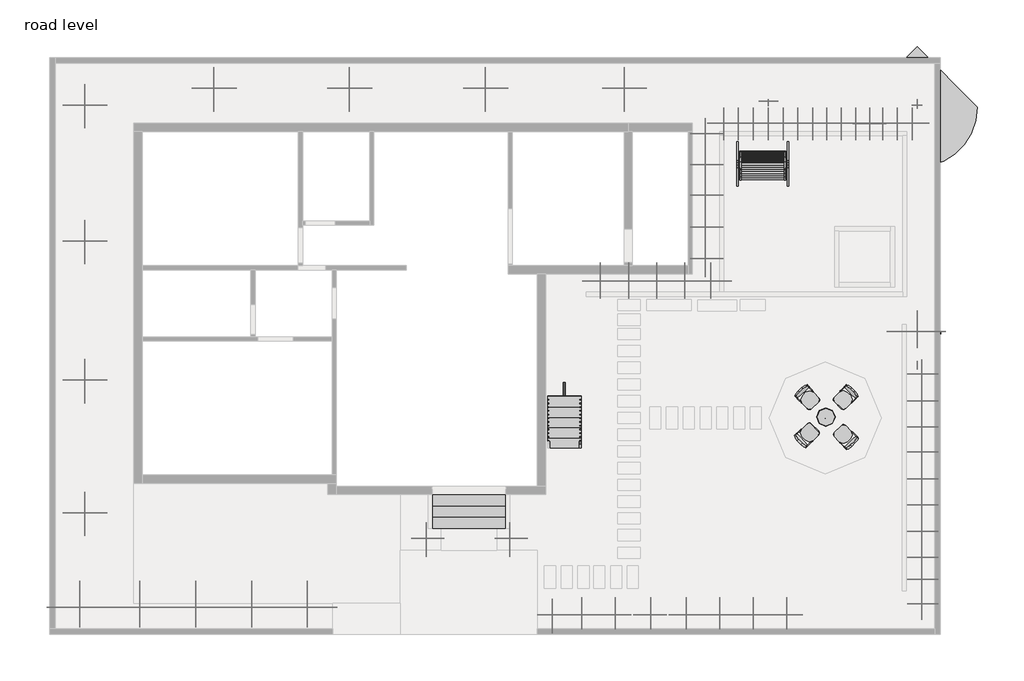
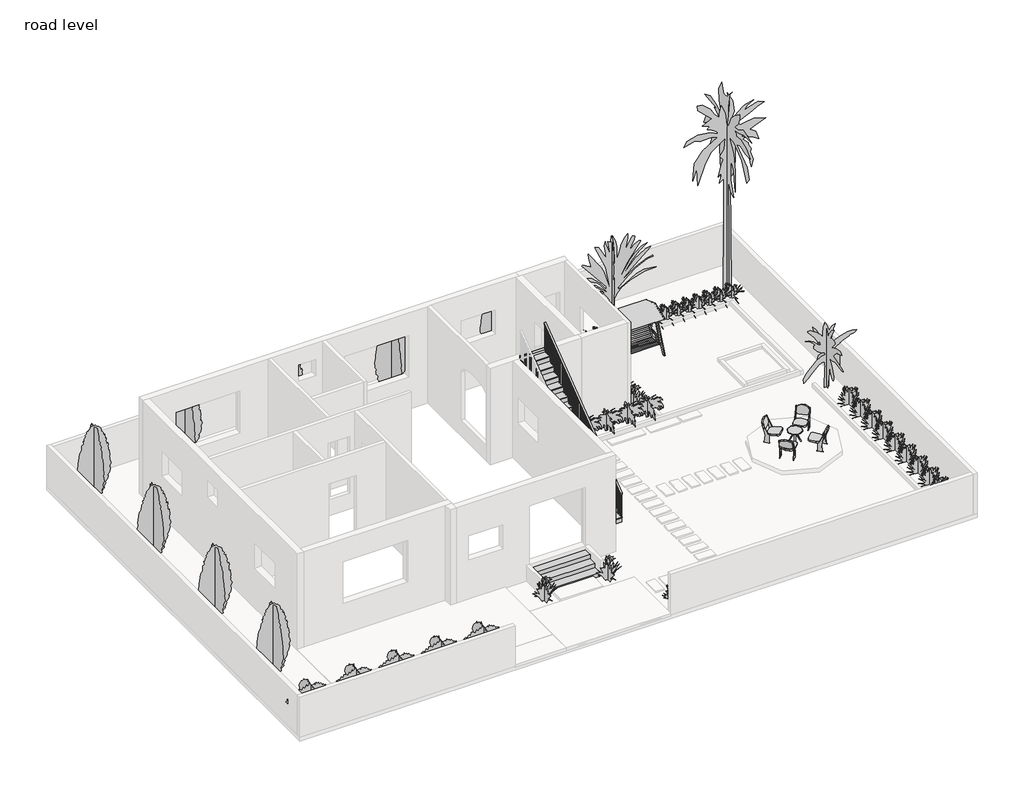
# One storey, part 3 of 3: 60 geographic elements, 7 furniture elements, 1 member, 1 railing, 1 stair flight.
"""IFC4 building model written with IfcOpenShell, lengths in millimetres."""

from ifc_helpers import new_model, si_unit, frame, origin, place, context, project, spatial, polyline, outline, extrude, transform, mapped, element, save
from components import furniture_0610_x_0160mm_a8fad5e2, casework_1_casework_1_50447f05, furniture_eb3a3c23, furniture_9d41381f, rpc_plant_tropical_55f6ff97, rpc_plant_tropical_6475341c, rpc_plant_tropical_agave_1_5_93a2a214, rpc_plant_tropical_dagger_2_80c14bd7, rpc_plant_tropical_japanese_fern_2_5_30b4c15b, rpc_plant_tropical_jungle_flame_3_9c4808c2, rpc_tree_deciduous_japanese_cherry_15_056c1364, rpc_tree_tropical_cuban_royal_palm_25_6f0ceb55, rpc_tree_tropical_japanese_fiber_banana_8_fc2fb2a9, rpc_tree_tropical_orange_tree_11_f00c8d58, stair_flight_3767e4ab

model = new_model("IFC4")

# Units and contexts
model_context = context("Model", 3, world=origin())
ifc_project = project(units=[si_unit("LENGTHUNIT", "METRE", prefix="MILLI")], contexts=[model_context])

# Site, building, storey
site = spatial("IfcSite", under=ifc_project)
building = spatial("IfcBuilding", under=site)
storey = spatial("IfcBuildingStorey", under=building, Name="road level", Elevation=0.0)

# Furniture
placement = place(None, origin())
furniture_0610_x_0160mm_shape = furniture_0610_x_0160mm_a8fad5e2(model_context)
element("IfcFurniture", 1, ObjectType="0610 x 0160mm", at=placement, inside=storey, context=model_context, shape_type="MappedRepresentation", body=[
    mapped(furniture_0610_x_0160mm_shape, transform((-1316.0822975, 10572.2724647, 0.0), x_axis=(1.0, 0.0, 0.0), y_axis=(0.0, 1.0, 0.0), z_axis=(0.0, 0.0, 1.0))),
])
casework_1_casework_1_shape = casework_1_casework_1_50447f05(model_context)
element("IfcFurniture", 2, ObjectType="Casework 1 : Casework 1", at=placement, inside=storey, context=model_context, shape_type="MappedRepresentation", body=[
    mapped(casework_1_casework_1_shape, transform((0.0, 0.0, 0.0), x_axis=(1.0, 0.0, 0.0), y_axis=(0.0, 1.0, 0.0), z_axis=(0.0, 0.0, 1.0))),
])
furniture_shape = furniture_eb3a3c23(model_context)
element("IfcFurniture", 3, ObjectType="Seating-Auditorium : 18\" x 24\" x 30\"", at=placement, inside=storey, context=model_context, shape_type="MappedRepresentation", body=[
    mapped(furniture_shape, transform((326.3169487, 5369.4995733, 152.4), x_axis=(-0.7331098777786673, -0.6801102168791081, 0.0), y_axis=(0.6801102168791081, -0.7331098777786673, 0.0), z_axis=(0.0, 0.0, 1.0))),
])
element("IfcFurniture", 4, ObjectType="Seating-Auditorium : 18\" x 24\" x 30\"", at=placement, inside=storey, context=model_context, shape_type="MappedRepresentation", body=[
    mapped(furniture_shape, transform((1406.8923034, 3783.3159111, 152.4), x_axis=(0.7169274118178623, 0.6971478223333565, 0.0), y_axis=(-0.6971478223333565, 0.7169274118178623, 0.0), z_axis=(0.0, 0.0, 1.0))),
])
element("IfcFurniture", 5, ObjectType="Seating-Auditorium : 18\" x 24\" x 30\"", at=placement, inside=storey, context=model_context, shape_type="MappedRepresentation", body=[
    mapped(furniture_shape, transform((1634.2545935, 5143.3486185, 152.4), x_axis=(-0.7104362628512833, 0.7037615479875996, 0.0), y_axis=(-0.7037615479875996, -0.7104362628512833, 0.0), z_axis=(0.0, 0.0, 1.0))),
])
element("IfcFurniture", 6, ObjectType="Seating-Auditorium : 18\" x 24\" x 30\"", at=placement, inside=storey, context=model_context, shape_type="MappedRepresentation", body=[
    mapped(furniture_shape, transform((76.4452405, 4067.2149284, 152.4), x_axis=(0.6883538503123506, -0.7253750593728473, 0.0), y_axis=(0.7253750593728473, 0.6883538503123506, 0.0), z_axis=(0.0, 0.0, 1.0))),
])
furniture_2_shape = furniture_9d41381f(model_context)
element("IfcFurniture", 7, ObjectType="Table-Trio End : 20\" Diameter", at=placement, inside=storey, context=model_context, shape_type="MappedRepresentation", body=[
    mapped(furniture_2_shape, transform((844.5582587, 4574.5465218, 152.4), x_axis=(1.0, 0.0, 0.0), y_axis=(0.0, 1.0, 0.0), z_axis=(0.0, 0.0, 1.0))),
])

# Geographic elements
rpc_plant_tropical_shape = rpc_plant_tropical_55f6ff97(model_context)
element("IfcGeographicElement", 8, ObjectType="RPC Plant - Tropical", at=placement, inside=storey, context=model_context, shape_type="MappedRepresentation", body=[
    mapped(rpc_plant_tropical_shape, transform((-7774.2983292, 1266.1965218, 0.0), x_axis=(1.0, 0.0, 0.0), y_axis=(0.0, 1.0, 0.0), z_axis=(0.0, 0.0, 1.0))),
])
element("IfcGeographicElement", 9, ObjectType="RPC Plant - Tropical", at=placement, inside=storey, context=model_context, shape_type="MappedRepresentation", body=[
    mapped(rpc_plant_tropical_shape, transform((-10048.7417413, 1266.1965218, 0.0), x_axis=(1.0, 0.0, 0.0), y_axis=(0.0, 1.0, 0.0), z_axis=(0.0, 0.0, 1.0))),
])
element("IfcGeographicElement", 10, ObjectType="RPC Plant - Tropical", at=placement, inside=storey, context=model_context, shape_type="MappedRepresentation", body=[
    mapped(rpc_plant_tropical_shape, transform((-2451.0917413, 12308.8465218, 0.0), x_axis=(1.0, 0.0, 0.0), y_axis=(0.0, 1.0, 0.0), z_axis=(0.0, 0.0, 1.0))),
])
element("IfcGeographicElement", 11, ObjectType="RPC Plant - Tropical", at=placement, inside=storey, context=model_context, shape_type="MappedRepresentation", body=[
    mapped(rpc_plant_tropical_shape, transform((-2451.0917413, 11470.6465218, 0.0), x_axis=(1.0, 0.0, 0.0), y_axis=(0.0, 1.0, 0.0), z_axis=(0.0, 0.0, 1.0))),
])
element("IfcGeographicElement", 12, ObjectType="RPC Plant - Tropical", at=placement, inside=storey, context=model_context, shape_type="MappedRepresentation", body=[
    mapped(rpc_plant_tropical_shape, transform((-2451.0917413, 10632.4465218, 0.0), x_axis=(1.0, 0.0, 0.0), y_axis=(0.0, 1.0, 0.0), z_axis=(0.0, 0.0, 1.0))),
])
element("IfcGeographicElement", 13, ObjectType="RPC Plant - Tropical", at=placement, inside=storey, context=model_context, shape_type="MappedRepresentation", body=[
    mapped(rpc_plant_tropical_shape, transform((-2451.0917413, 9762.4965218, 0.0), x_axis=(1.0, 0.0, 0.0), y_axis=(0.0, 1.0, 0.0), z_axis=(0.0, 0.0, 1.0))),
])
element("IfcGeographicElement", 14, ObjectType="RPC Plant - Tropical", at=placement, inside=storey, context=model_context, shape_type="MappedRepresentation", body=[
    mapped(rpc_plant_tropical_shape, transform((-2451.0917413, 8898.8965218, 0.0), x_axis=(1.0, 0.0, 0.0), y_axis=(0.0, 1.0, 0.0), z_axis=(0.0, 0.0, 1.0))),
])
element("IfcGeographicElement", 15, ObjectType="RPC Plant - Tropical", at=placement, inside=storey, context=model_context, shape_type="MappedRepresentation", body=[
    mapped(rpc_plant_tropical_shape, transform((-6623.0417413, -816.6034782, 0.0), x_axis=(1.0, 0.0, 0.0), y_axis=(0.0, 1.0, 0.0), z_axis=(0.0, 0.0, 1.0))),
])
rpc_plant_tropical_2_shape = rpc_plant_tropical_6475341c(model_context)
element("IfcGeographicElement", 16, ObjectType="RPC Plant - Tropical", at=placement, inside=storey, context=model_context, shape_type="MappedRepresentation", body=[
    mapped(rpc_plant_tropical_2_shape, transform((-13233.3917413, -613.4034782, 0.0), x_axis=(1.0, 0.0, 0.0), y_axis=(0.0, 1.0, 0.0), z_axis=(0.0, 0.0, 1.0))),
])
element("IfcGeographicElement", 17, ObjectType="RPC Plant - Tropical", at=placement, inside=storey, context=model_context, shape_type="MappedRepresentation", body=[
    mapped(rpc_plant_tropical_2_shape, transform((-14757.3917413, -613.4034782, 0.0), x_axis=(1.0, 0.0, 0.0), y_axis=(0.0, 1.0, 0.0), z_axis=(0.0, 0.0, 1.0))),
])
element("IfcGeographicElement", 18, ObjectType="RPC Plant - Tropical", at=placement, inside=storey, context=model_context, shape_type="MappedRepresentation", body=[
    mapped(rpc_plant_tropical_2_shape, transform((-16281.3917413, -613.4034782, 0.0), x_axis=(1.0, 0.0, 0.0), y_axis=(0.0, 1.0, 0.0), z_axis=(0.0, 0.0, 1.0))),
])
element("IfcGeographicElement", 19, ObjectType="RPC Plant - Tropical", at=placement, inside=storey, context=model_context, shape_type="MappedRepresentation", body=[
    mapped(rpc_plant_tropical_2_shape, transform((-17805.3917413, -613.4034782, 0.0), x_axis=(1.0, 0.0, 0.0), y_axis=(0.0, 1.0, 0.0), z_axis=(0.0, 0.0, 1.0))),
])
element("IfcGeographicElement", 20, ObjectType="RPC Plant - Tropical", at=placement, inside=storey, context=model_context, shape_type="MappedRepresentation", body=[
    mapped(rpc_plant_tropical_2_shape, transform((-19443.6917413, -613.4034782, 0.0), x_axis=(1.0, 0.0, 0.0), y_axis=(0.0, 1.0, 0.0), z_axis=(0.0, 0.0, 1.0))),
])
rpc_plant_tropical_agave_1_5_shape = rpc_plant_tropical_agave_1_5_93a2a214(model_context)
element("IfcGeographicElement", 21, ObjectType="RPC Plant - Tropical : Agave - 1.5'", at=placement, inside=storey, context=model_context, shape_type="MappedRepresentation", body=[
    mapped(rpc_plant_tropical_agave_1_5_shape, transform((-1936.7417413, 12594.5965218, 0.0), x_axis=(1.0, 0.0, 0.0), y_axis=(0.0, 1.0, 0.0), z_axis=(0.0, 0.0, 1.0))),
])
element("IfcGeographicElement", 22, ObjectType="RPC Plant - Tropical : Agave - 1.5'", at=placement, inside=storey, context=model_context, shape_type="MappedRepresentation", body=[
    mapped(rpc_plant_tropical_agave_1_5_shape, transform((-1543.0417413, 12594.5965218, 0.0), x_axis=(1.0, 0.0, 0.0), y_axis=(0.0, 1.0, 0.0), z_axis=(0.0, 0.0, 1.0))),
])
element("IfcGeographicElement", 23, ObjectType="RPC Plant - Tropical : Agave - 1.5'", at=placement, inside=storey, context=model_context, shape_type="MappedRepresentation", body=[
    mapped(rpc_plant_tropical_agave_1_5_shape, transform((-1136.6417413, 12594.5965218, 0.0), x_axis=(1.0, 0.0, 0.0), y_axis=(0.0, 1.0, 0.0), z_axis=(0.0, 0.0, 1.0))),
])
element("IfcGeographicElement", 24, ObjectType="RPC Plant - Tropical : Agave - 1.5'", at=placement, inside=storey, context=model_context, shape_type="MappedRepresentation", body=[
    mapped(rpc_plant_tropical_agave_1_5_shape, transform((-730.2417413, 12594.5965218, 0.0), x_axis=(1.0, 0.0, 0.0), y_axis=(0.0, 1.0, 0.0), z_axis=(0.0, 0.0, 1.0))),
])
element("IfcGeographicElement", 25, ObjectType="RPC Plant - Tropical : Agave - 1.5'", at=placement, inside=storey, context=model_context, shape_type="MappedRepresentation", body=[
    mapped(rpc_plant_tropical_agave_1_5_shape, transform((-323.8417413, 12594.5965218, 0.0), x_axis=(1.0, 0.0, 0.0), y_axis=(0.0, 1.0, 0.0), z_axis=(0.0, 0.0, 1.0))),
])
element("IfcGeographicElement", 26, ObjectType="RPC Plant - Tropical : Agave - 1.5'", at=placement, inside=storey, context=model_context, shape_type="MappedRepresentation", body=[
    mapped(rpc_plant_tropical_agave_1_5_shape, transform((869.9582587, 12594.5965218, 0.0), x_axis=(1.0, 0.0, 0.0), y_axis=(0.0, 1.0, 0.0), z_axis=(0.0, 0.0, 1.0))),
])
element("IfcGeographicElement", 27, ObjectType="RPC Plant - Tropical : Agave - 1.5'", at=placement, inside=storey, context=model_context, shape_type="MappedRepresentation", body=[
    mapped(rpc_plant_tropical_agave_1_5_shape, transform((488.9582587, 12594.5965218, 0.0), x_axis=(1.0, 0.0, 0.0), y_axis=(0.0, 1.0, 0.0), z_axis=(0.0, 0.0, 1.0))),
])
element("IfcGeographicElement", 28, ObjectType="RPC Plant - Tropical : Agave - 1.5'", at=placement, inside=storey, context=model_context, shape_type="MappedRepresentation", body=[
    mapped(rpc_plant_tropical_agave_1_5_shape, transform((82.5582587, 12594.5965218, 0.0), x_axis=(1.0, 0.0, 0.0), y_axis=(0.0, 1.0, 0.0), z_axis=(0.0, 0.0, 1.0))),
])
element("IfcGeographicElement", 29, ObjectType="RPC Plant - Tropical : Agave - 1.5'", at=placement, inside=storey, context=model_context, shape_type="MappedRepresentation", body=[
    mapped(rpc_plant_tropical_agave_1_5_shape, transform((1270.0082587, 12594.5965218, 0.0), x_axis=(1.0, 0.0, 0.0), y_axis=(0.0, 1.0, 0.0), z_axis=(0.0, 0.0, 1.0))),
])
element("IfcGeographicElement", 30, ObjectType="RPC Plant - Tropical : Agave - 1.5'", at=placement, inside=storey, context=model_context, shape_type="MappedRepresentation", body=[
    mapped(rpc_plant_tropical_agave_1_5_shape, transform((2036.1358852, 12588.3418094, 0.0), x_axis=(1.0, 0.0, 0.0), y_axis=(0.0, 1.0, 0.0), z_axis=(0.0, 0.0, 1.0))),
])
element("IfcGeographicElement", 31, ObjectType="RPC Plant - Tropical : Agave - 1.5'", at=placement, inside=storey, context=model_context, shape_type="MappedRepresentation", body=[
    mapped(rpc_plant_tropical_agave_1_5_shape, transform((1657.3582587, 12594.5965218, 0.0), x_axis=(1.0, 0.0, 0.0), y_axis=(0.0, 1.0, 0.0), z_axis=(0.0, 0.0, 1.0))),
])
element("IfcGeographicElement", 32, ObjectType="RPC Plant - Tropical : Agave - 1.5'", at=placement, inside=storey, context=model_context, shape_type="MappedRepresentation", body=[
    mapped(rpc_plant_tropical_agave_1_5_shape, transform((2393.9582587, 12594.5965218, 0.0), x_axis=(1.0, 0.0, 0.0), y_axis=(0.0, 1.0, 0.0), z_axis=(0.0, 0.0, 1.0))),
])
element("IfcGeographicElement", 33, ObjectType="RPC Plant - Tropical : Agave - 1.5'", at=placement, inside=storey, context=model_context, shape_type="MappedRepresentation", body=[
    mapped(rpc_plant_tropical_agave_1_5_shape, transform((2785.3590161, 12594.5965218, 0.0), x_axis=(1.0, 0.0, 0.0), y_axis=(0.0, 1.0, 0.0), z_axis=(0.0, 0.0, 1.0))),
])
element("IfcGeographicElement", 34, ObjectType="RPC Plant - Tropical : Agave - 1.5'", at=placement, inside=storey, context=model_context, shape_type="MappedRepresentation", body=[
    mapped(rpc_plant_tropical_agave_1_5_shape, transform((3200.4082587, 12594.5965218, 0.0), x_axis=(1.0, 0.0, 0.0), y_axis=(0.0, 1.0, 0.0), z_axis=(0.0, 0.0, 1.0))),
])
rpc_plant_tropical_dagger_2_shape = rpc_plant_tropical_dagger_2_80c14bd7(model_context)
element("IfcGeographicElement", 35, ObjectType="RPC Plant - Tropical : Dagger - 2'", at=placement, inside=storey, context=model_context, shape_type="MappedRepresentation", body=[
    mapped(rpc_plant_tropical_dagger_2_shape, transform((3460.7582587, 5755.6465218, 0.0), x_axis=(1.0, 0.0, 0.0), y_axis=(0.0, 1.0, 0.0), z_axis=(0.0, 0.0, 1.0))),
])
element("IfcGeographicElement", 36, ObjectType="RPC Plant - Tropical : Dagger - 2'", at=placement, inside=storey, context=model_context, shape_type="MappedRepresentation", body=[
    mapped(rpc_plant_tropical_dagger_2_shape, transform((3460.7582587, 5019.0465218, 0.0), x_axis=(1.0, 0.0, 0.0), y_axis=(0.0, 1.0, 0.0), z_axis=(0.0, 0.0, 1.0))),
])
element("IfcGeographicElement", 37, ObjectType="RPC Plant - Tropical : Dagger - 2'", at=placement, inside=storey, context=model_context, shape_type="MappedRepresentation", body=[
    mapped(rpc_plant_tropical_dagger_2_shape, transform((3460.7582587, 4307.8465218, 0.0), x_axis=(1.0, 0.0, 0.0), y_axis=(0.0, 1.0, 0.0), z_axis=(0.0, 0.0, 1.0))),
])
element("IfcGeographicElement", 38, ObjectType="RPC Plant - Tropical : Dagger - 2'", at=placement, inside=storey, context=model_context, shape_type="MappedRepresentation", body=[
    mapped(rpc_plant_tropical_dagger_2_shape, transform((3460.7582587, 3622.0465218, 0.0), x_axis=(1.0, 0.0, 0.0), y_axis=(0.0, 1.0, 0.0), z_axis=(0.0, 0.0, 1.0))),
])
element("IfcGeographicElement", 39, ObjectType="RPC Plant - Tropical : Dagger - 2'", at=placement, inside=storey, context=model_context, shape_type="MappedRepresentation", body=[
    mapped(rpc_plant_tropical_dagger_2_shape, transform((3460.7582587, 2885.4465218, 0.0), x_axis=(1.0, 0.0, 0.0), y_axis=(0.0, 1.0, 0.0), z_axis=(0.0, 0.0, 1.0))),
])
element("IfcGeographicElement", 40, ObjectType="RPC Plant - Tropical : Dagger - 2'", at=placement, inside=storey, context=model_context, shape_type="MappedRepresentation", body=[
    mapped(rpc_plant_tropical_dagger_2_shape, transform((3460.7582587, 2174.2465218, 0.0), x_axis=(1.0, 0.0, 0.0), y_axis=(0.0, 1.0, 0.0), z_axis=(0.0, 0.0, 1.0))),
])
element("IfcGeographicElement", 41, ObjectType="RPC Plant - Tropical : Dagger - 2'", at=placement, inside=storey, context=model_context, shape_type="MappedRepresentation", body=[
    mapped(rpc_plant_tropical_dagger_2_shape, transform((3460.7582587, 1463.0465218, 0.0), x_axis=(1.0, 0.0, 0.0), y_axis=(0.0, 1.0, 0.0), z_axis=(0.0, 0.0, 1.0))),
])
element("IfcGeographicElement", 42, ObjectType="RPC Plant - Tropical : Dagger - 2'", at=placement, inside=storey, context=model_context, shape_type="MappedRepresentation", body=[
    mapped(rpc_plant_tropical_dagger_2_shape, transform((3460.7582587, 751.8465218, 0.0), x_axis=(1.0, 0.0, 0.0), y_axis=(0.0, 1.0, 0.0), z_axis=(0.0, 0.0, 1.0))),
])
element("IfcGeographicElement", 43, ObjectType="RPC Plant - Tropical : Dagger - 2'", at=placement, inside=storey, context=model_context, shape_type="MappedRepresentation", body=[
    mapped(rpc_plant_tropical_dagger_2_shape, transform((3460.7582587, 142.2465218, 0.0), x_axis=(1.0, 0.0, 0.0), y_axis=(0.0, 1.0, 0.0), z_axis=(0.0, 0.0, 1.0))),
])
element("IfcGeographicElement", 44, ObjectType="RPC Plant - Tropical : Dagger - 2'", at=placement, inside=storey, context=model_context, shape_type="MappedRepresentation", body=[
    mapped(rpc_plant_tropical_dagger_2_shape, transform((3460.7582587, -514.2328583, 0.0), x_axis=(1.0, 0.0, 0.0), y_axis=(0.0, 1.0, 0.0), z_axis=(0.0, 0.0, 1.0))),
])
rpc_plant_tropical_japanese_fern_2_5_shape = rpc_plant_tropical_japanese_fern_2_5_30b4c15b(model_context)
element("IfcGeographicElement", 45, ObjectType="RPC Plant - Tropical : Japanese Fern - 2.5'", at=placement, inside=storey, context=model_context, shape_type="MappedRepresentation", body=[
    mapped(rpc_plant_tropical_japanese_fern_2_5_shape, transform((-5308.5917413, 8289.2965218, 0.0), x_axis=(1.0, 0.0, 0.0), y_axis=(0.0, 1.0, 0.0), z_axis=(0.0, 0.0, 1.0))),
])
element("IfcGeographicElement", 46, ObjectType="RPC Plant - Tropical : Japanese Fern - 2.5'", at=placement, inside=storey, context=model_context, shape_type="MappedRepresentation", body=[
    mapped(rpc_plant_tropical_japanese_fern_2_5_shape, transform((-3765.5417413, 8289.2965218, 0.0), x_axis=(1.0, 0.0, 0.0), y_axis=(0.0, 1.0, 0.0), z_axis=(0.0, 0.0, 1.0))),
])
element("IfcGeographicElement", 47, ObjectType="RPC Plant - Tropical : Japanese Fern - 2.5'", at=placement, inside=storey, context=model_context, shape_type="MappedRepresentation", body=[
    mapped(rpc_plant_tropical_japanese_fern_2_5_shape, transform((-4527.5417413, 8289.2965218, 0.0), x_axis=(1.0, 0.0, 0.0), y_axis=(0.0, 1.0, 0.0), z_axis=(0.0, 0.0, 1.0))),
])
element("IfcGeographicElement", 48, ObjectType="RPC Plant - Tropical : Japanese Fern - 2.5'", at=placement, inside=storey, context=model_context, shape_type="MappedRepresentation", body=[
    mapped(rpc_plant_tropical_japanese_fern_2_5_shape, transform((-3003.5417413, 8289.2965218, 0.0), x_axis=(1.0, 0.0, 0.0), y_axis=(0.0, 1.0, 0.0), z_axis=(0.0, 0.0, 1.0))),
])
element("IfcGeographicElement", 49, ObjectType="RPC Plant - Tropical : Japanese Fern - 2.5'", at=placement, inside=storey, context=model_context, shape_type="MappedRepresentation", body=[
    mapped(rpc_plant_tropical_japanese_fern_2_5_shape, transform((-2298.6917413, 8289.2965218, 0.0), x_axis=(1.0, 0.0, 0.0), y_axis=(0.0, 1.0, 0.0), z_axis=(0.0, 0.0, 1.0))),
])
rpc_plant_tropical_jungle_flame_3_shape = rpc_plant_tropical_jungle_flame_3_9c4808c2(model_context)
element("IfcGeographicElement", 50, ObjectType="RPC Plant - Tropical : Jungle Flame - 3'", at=placement, inside=storey, context=model_context, shape_type="MappedRepresentation", body=[
    mapped(rpc_plant_tropical_jungle_flame_3_shape, transform((-222.2417413, -816.6034782, 0.0), x_axis=(1.0, 0.0, 0.0), y_axis=(0.0, 1.0, 0.0), z_axis=(0.0, 0.0, 1.0))),
])
element("IfcGeographicElement", 51, ObjectType="RPC Plant - Tropical : Jungle Flame - 3'", at=placement, inside=storey, context=model_context, shape_type="MappedRepresentation", body=[
    mapped(rpc_plant_tropical_jungle_flame_3_shape, transform((-1136.6417413, -816.6034782, 0.0), x_axis=(1.0, 0.0, 0.0), y_axis=(0.0, 1.0, 0.0), z_axis=(0.0, 0.0, 1.0))),
])
element("IfcGeographicElement", 52, ObjectType="RPC Plant - Tropical : Jungle Flame - 3'", at=placement, inside=storey, context=model_context, shape_type="MappedRepresentation", body=[
    mapped(rpc_plant_tropical_jungle_flame_3_shape, transform((-2051.0417413, -816.6034782, 0.0), x_axis=(1.0, 0.0, 0.0), y_axis=(0.0, 1.0, 0.0), z_axis=(0.0, 0.0, 1.0))),
])
element("IfcGeographicElement", 53, ObjectType="RPC Plant - Tropical : Jungle Flame - 3'", at=placement, inside=storey, context=model_context, shape_type="MappedRepresentation", body=[
    mapped(rpc_plant_tropical_jungle_flame_3_shape, transform((-2965.4417413, -816.6034782, 0.0), x_axis=(1.0, 0.0, 0.0), y_axis=(0.0, 1.0, 0.0), z_axis=(0.0, 0.0, 1.0))),
])
element("IfcGeographicElement", 54, ObjectType="RPC Plant - Tropical : Jungle Flame - 3'", at=placement, inside=storey, context=model_context, shape_type="MappedRepresentation", body=[
    mapped(rpc_plant_tropical_jungle_flame_3_shape, transform((-3930.6417413, -816.6034782, 0.0), x_axis=(1.0, 0.0, 0.0), y_axis=(0.0, 1.0, 0.0), z_axis=(0.0, 0.0, 1.0))),
])
element("IfcGeographicElement", 55, ObjectType="RPC Plant - Tropical : Jungle Flame - 3'", at=placement, inside=storey, context=model_context, shape_type="MappedRepresentation", body=[
    mapped(rpc_plant_tropical_jungle_flame_3_shape, transform((-4895.8417413, -816.6034782, 0.0), x_axis=(1.0, 0.0, 0.0), y_axis=(0.0, 1.0, 0.0), z_axis=(0.0, 0.0, 1.0))),
])
element("IfcGeographicElement", 56, ObjectType="RPC Plant - Tropical : Jungle Flame - 3'", at=placement, inside=storey, context=model_context, shape_type="MappedRepresentation", body=[
    mapped(rpc_plant_tropical_jungle_flame_3_shape, transform((-5810.2417413, -816.6034782, 0.0), x_axis=(1.0, 0.0, 0.0), y_axis=(0.0, 1.0, 0.0), z_axis=(0.0, 0.0, 1.0))),
])
rpc_tree_deciduous_japanese_cherry_15_shape = rpc_tree_deciduous_japanese_cherry_15_056c1364(model_context)
element("IfcGeographicElement", 57, ObjectType="RPC Tree - Deciduous : Japanese Cherry - 15'", at=placement, inside=storey, context=model_context, shape_type="MappedRepresentation", body=[
    mapped(rpc_tree_deciduous_japanese_cherry_15_shape, transform((-19367.4917413, 5584.1965218, 0.0), x_axis=(1.0, 0.0, 0.0), y_axis=(0.0, 1.0, 0.0), z_axis=(0.0, 0.0, 1.0))),
])
element("IfcGeographicElement", 58, ObjectType="RPC Tree - Deciduous : Japanese Cherry - 15'", at=placement, inside=storey, context=model_context, shape_type="MappedRepresentation", body=[
    mapped(rpc_tree_deciduous_japanese_cherry_15_shape, transform((-19367.4917413, 9381.4965218, 0.0), x_axis=(1.0, 0.0, 0.0), y_axis=(0.0, 1.0, 0.0), z_axis=(0.0, 0.0, 1.0))),
])
element("IfcGeographicElement", 59, ObjectType="RPC Tree - Deciduous : Japanese Cherry - 15'", at=placement, inside=storey, context=model_context, shape_type="MappedRepresentation", body=[
    mapped(rpc_tree_deciduous_japanese_cherry_15_shape, transform((-19367.4917413, 1964.6965218, 0.0), x_axis=(1.0, 0.0, 0.0), y_axis=(0.0, 1.0, 0.0), z_axis=(0.0, 0.0, 1.0))),
])
element("IfcGeographicElement", 60, ObjectType="RPC Tree - Deciduous : Japanese Cherry - 15'", at=placement, inside=storey, context=model_context, shape_type="MappedRepresentation", body=[
    mapped(rpc_tree_deciduous_japanese_cherry_15_shape, transform((-19367.4917413, 13089.8965218, 0.0), x_axis=(1.0, 0.0, 0.0), y_axis=(0.0, 1.0, 0.0), z_axis=(0.0, 0.0, 1.0))),
])
element("IfcGeographicElement", 61, ObjectType="RPC Tree - Deciduous : Japanese Cherry - 15'", at=placement, inside=storey, context=model_context, shape_type="MappedRepresentation", body=[
    mapped(rpc_tree_deciduous_japanese_cherry_15_shape, transform((-15843.2417413, 13547.0965218, 0.0), x_axis=(1.0, 0.0, 0.0), y_axis=(0.0, 1.0, 0.0), z_axis=(0.0, 0.0, 1.0))),
])
element("IfcGeographicElement", 62, ObjectType="RPC Tree - Deciduous : Japanese Cherry - 15'", at=placement, inside=storey, context=model_context, shape_type="MappedRepresentation", body=[
    mapped(rpc_tree_deciduous_japanese_cherry_15_shape, transform((-12147.5417413, 13547.0965218, 0.0), x_axis=(1.0, 0.0, 0.0), y_axis=(0.0, 1.0, 0.0), z_axis=(0.0, 0.0, 1.0))),
])
element("IfcGeographicElement", 63, ObjectType="RPC Tree - Deciduous : Japanese Cherry - 15'", at=placement, inside=storey, context=model_context, shape_type="MappedRepresentation", body=[
    mapped(rpc_tree_deciduous_japanese_cherry_15_shape, transform((-8441.0483292, 13547.0965218, 0.0), x_axis=(1.0, 0.0, 0.0), y_axis=(0.0, 1.0, 0.0), z_axis=(0.0, 0.0, 1.0))),
])
element("IfcGeographicElement", 64, ObjectType="RPC Tree - Deciduous : Japanese Cherry - 15'", at=placement, inside=storey, context=model_context, shape_type="MappedRepresentation", body=[
    mapped(rpc_tree_deciduous_japanese_cherry_15_shape, transform((-4660.8917413, 13547.0965218, 0.0), x_axis=(1.0, 0.0, 0.0), y_axis=(0.0, 1.0, 0.0), z_axis=(0.0, 0.0, 1.0))),
])
rpc_tree_tropical_cuban_royal_palm_25_shape = rpc_tree_tropical_cuban_royal_palm_25_6f0ceb55(model_context)
element("IfcGeographicElement", 65, ObjectType="RPC Tree - Tropical : Cuban Royal Palm - 25'", at=placement, inside=storey, context=model_context, shape_type="MappedRepresentation", body=[
    mapped(rpc_tree_tropical_cuban_royal_palm_25_shape, transform((3333.7582587, 13089.8965218, 0.0), x_axis=(1.0, 0.0, 0.0), y_axis=(0.0, 1.0, 0.0), z_axis=(0.0, 0.0, 1.0))),
])
rpc_tree_tropical_japanese_fiber_banana_8_shape = rpc_tree_tropical_japanese_fiber_banana_8_fc2fb2a9(model_context)
element("IfcGeographicElement", 66, ObjectType="RPC Tree - Tropical : Japanese Fiber Banana - 8'", at=placement, inside=storey, context=model_context, shape_type="MappedRepresentation", body=[
    mapped(rpc_tree_tropical_japanese_fiber_banana_8_shape, transform((3333.7582587, 6911.3465218, 0.0), x_axis=(1.0, 0.0, 0.0), y_axis=(0.0, 1.0, 0.0), z_axis=(0.0, 0.0, 1.0))),
])
rpc_tree_tropical_orange_tree_11_shape = rpc_tree_tropical_orange_tree_11_f00c8d58(model_context)
element("IfcGeographicElement", 67, ObjectType="RPC Tree - Tropical : Orange Tree - 11'", at=placement, inside=storey, context=model_context, shape_type="MappedRepresentation", body=[
    mapped(rpc_tree_tropical_orange_tree_11_shape, transform((-730.2417413, 13191.4965218, 0.0), x_axis=(1.0, 0.0, 0.0), y_axis=(0.0, 1.0, 0.0), z_axis=(0.0, 0.0, 1.0))),
])

# Member
element("IfcMember", 68, ObjectType="Carriage - 2\" Width", at=placement, inside=storey, context=model_context, shape_type="SweptSolid", body=[
    extrude(outline(polyline([(8480.0992417, 3547.5333333), (8480.0992417, 3443.8157371), (3934.2624688, 0.0), (3762.0492417, 0.0), (3762.0492417, 160.8666667), (4041.4492417, 160.8666667), (4041.4492417, 372.5333333), (4320.8492417, 372.5333333), (4320.8492417, 584.2), (4600.2492417, 584.2), (4600.2492417, 795.8666667), (4879.6492417, 795.8666667), (4879.6492417, 1007.5333333), (5159.0492417, 1007.5333333), (5159.0492417, 1219.2), (5438.4492417, 1219.2), (5438.4492417, 1430.8666667), (5717.8492417, 1430.8666667), (5717.8492417, 1642.5333333), (5997.2492417, 1642.5333333), (5997.2492417, 1854.2), (6276.6492417, 1854.2), (6276.6492417, 2065.8666667), (6556.0492417, 2065.8666667), (6556.0492417, 2277.5333333), (6835.4492417, 2277.5333333), (6835.4492417, 2489.2), (7114.8492417, 2489.2), (7114.8492417, 2700.8666667), (7394.2492417, 2700.8666667), (7394.2492417, 2912.5333333), (7673.6492417, 2912.5333333), (7673.6492417, 3124.2), (7953.0492417, 3124.2), (7953.0492417, 3335.8666667), (8232.4492417, 3335.8666667), (8232.4492417, 3547.5333333), (8480.0992417, 3547.5333333)])), frame((-6311.8917413, 0.0, 0.0), z_axis=(1.0, 0.0, 0.0), x_axis=(0.0, 1.0, 0.0)), (0.0, 0.0, 1.0), 50.8),
])

# Railing
element("IfcRailing", 69, ObjectType="Handrail - Rectangular", at=placement, inside=storey, context=model_context, shape_type="SweptSolid", body=[
    extrude(outline(polyline([(3730.2992417, 1062.3350139), (3730.2992417, 1126.0666667), (8480.0992417, 4724.4), (8480.0992417, 4660.6683472), (3730.2992417, 1062.3350139)])), frame((-5880.0917413, 0.0, 0.0), z_axis=(1.0, 0.0, 0.0), x_axis=(0.0, 1.0, 0.0)), (0.0, 0.0, 1.0), 50.8),
    extrude(outline(polyline([(8394.3742417, 4595.7251654), (8413.4242417, 4610.1569836), (8413.4242417, 3598.3333333), (8394.3742417, 3598.3333333), (8394.3742417, 4595.7251654)])), frame((-5864.2167413, 0.0, 0.0), z_axis=(1.0, 0.0, 0.0), x_axis=(0.0, 1.0, 0.0)), (0.0, 0.0, 1.0), 19.05),
    extrude(outline(polyline([(8292.7742417, 4518.7554685), (8311.8242417, 4533.1872866), (8311.8242417, 3598.3333333), (8292.7742417, 3598.3333333), (8292.7742417, 4518.7554685)])), frame((-5864.2167413, 0.0, 0.0), z_axis=(1.0, 0.0, 0.0), x_axis=(0.0, 1.0, 0.0)), (0.0, 0.0, 1.0), 19.05),
    extrude(outline(polyline([(8191.1742417, 4441.7857715), (8210.2242417, 4456.2175897), (8210.2242417, 3598.3333333), (8191.1742417, 3598.3333333), (8191.1742417, 4441.7857715)])), frame((-5864.2167413, 0.0, 0.0), z_axis=(1.0, 0.0, 0.0), x_axis=(0.0, 1.0, 0.0)), (0.0, 0.0, 1.0), 19.05),
    extrude(outline(polyline([(8089.5742417, 4364.8160745), (8108.6242417, 4379.2478927), (8108.6242417, 3386.6666667), (8089.5742417, 3386.6666667), (8089.5742417, 4364.8160745)])), frame((-5864.2167413, 0.0, 0.0), z_axis=(1.0, 0.0, 0.0), x_axis=(0.0, 1.0, 0.0)), (0.0, 0.0, 1.0), 19.05),
    extrude(outline(polyline([(7987.9742417, 4287.8463775), (8007.0242417, 4302.2781957), (8007.0242417, 3386.6666667), (7987.9742417, 3386.6666667), (7987.9742417, 4287.8463775)])), frame((-5864.2167413, 0.0, 0.0), z_axis=(1.0, 0.0, 0.0), x_axis=(0.0, 1.0, 0.0)), (0.0, 0.0, 1.0), 19.05),
    extrude(outline(polyline([(7886.3742417, 4210.8766806), (7905.4242417, 4225.3084988), (7905.4242417, 3175.0), (7886.3742417, 3175.0), (7886.3742417, 4210.8766806)])), frame((-5864.2167413, 0.0, 0.0), z_axis=(1.0, 0.0, 0.0), x_axis=(0.0, 1.0, 0.0)), (0.0, 0.0, 1.0), 19.05),
    extrude(outline(polyline([(7784.7742417, 4133.9069836), (7803.8242417, 4148.3388018), (7803.8242417, 3175.0), (7784.7742417, 3175.0), (7784.7742417, 4133.9069836)])), frame((-5864.2167413, 0.0, 0.0), z_axis=(1.0, 0.0, 0.0), x_axis=(0.0, 1.0, 0.0)), (0.0, 0.0, 1.0), 19.05),
    extrude(outline(polyline([(7683.1742417, 4056.9372866), (7702.2242417, 4071.3691048), (7702.2242417, 3175.0), (7683.1742417, 3175.0), (7683.1742417, 4056.9372866)])), frame((-5864.2167413, 0.0, 0.0), z_axis=(1.0, 0.0, 0.0), x_axis=(0.0, 1.0, 0.0)), (0.0, 0.0, 1.0), 19.05),
    extrude(outline(polyline([(7581.5742417, 3979.9675897), (7600.6242417, 3994.3994079), (7600.6242417, 2963.3333333), (7581.5742417, 2963.3333333), (7581.5742417, 3979.9675897)])), frame((-5864.2167413, 0.0, 0.0), z_axis=(1.0, 0.0, 0.0), x_axis=(0.0, 1.0, 0.0)), (0.0, 0.0, 1.0), 19.05),
    extrude(outline(polyline([(7479.9742417, 3902.9978927), (7499.0242417, 3917.4297109), (7499.0242417, 2963.3333333), (7479.9742417, 2963.3333333), (7479.9742417, 3902.9978927)])), frame((-5864.2167413, 0.0, 0.0), z_axis=(1.0, 0.0, 0.0), x_axis=(0.0, 1.0, 0.0)), (0.0, 0.0, 1.0), 19.05),
    extrude(outline(polyline([(7378.3742417, 3826.0281957), (7397.4242417, 3840.4600139), (7397.4242417, 2963.3333333), (7378.3742417, 2963.3333333), (7378.3742417, 3826.0281957)])), frame((-5864.2167413, 0.0, 0.0), z_axis=(1.0, 0.0, 0.0), x_axis=(0.0, 1.0, 0.0)), (0.0, 0.0, 1.0), 19.05),
    extrude(outline(polyline([(7276.7742417, 3749.0584988), (7295.8242417, 3763.4903169), (7295.8242417, 2751.6666667), (7276.7742417, 2751.6666667), (7276.7742417, 3749.0584988)])), frame((-5864.2167413, 0.0, 0.0), z_axis=(1.0, 0.0, 0.0), x_axis=(0.0, 1.0, 0.0)), (0.0, 0.0, 1.0), 19.05),
    extrude(outline(polyline([(7175.1742417, 3672.0888018), (7194.2242417, 3686.52062), (7194.2242417, 2751.6666667), (7175.1742417, 2751.6666667), (7175.1742417, 3672.0888018)])), frame((-5864.2167413, 0.0, 0.0), z_axis=(1.0, 0.0, 0.0), x_axis=(0.0, 1.0, 0.0)), (0.0, 0.0, 1.0), 19.05),
    extrude(outline(polyline([(7073.5742417, 3595.1191048), (7092.6242417, 3609.550923), (7092.6242417, 2751.6666667), (7073.5742417, 2751.6666667), (7073.5742417, 3595.1191048)])), frame((-5864.2167413, 0.0, 0.0), z_axis=(1.0, 0.0, 0.0), x_axis=(0.0, 1.0, 0.0)), (0.0, 0.0, 1.0), 19.05),
    extrude(outline(polyline([(6971.9742417, 3518.1494079), (6991.0242417, 3532.581226), (6991.0242417, 2540.0), (6971.9742417, 2540.0), (6971.9742417, 3518.1494079)])), frame((-5864.2167413, 0.0, 0.0), z_axis=(1.0, 0.0, 0.0), x_axis=(0.0, 1.0, 0.0)), (0.0, 0.0, 1.0), 19.05),
    extrude(outline(polyline([(6870.3742417, 3441.1797109), (6889.4242417, 3455.6115291), (6889.4242417, 2540.0), (6870.3742417, 2540.0), (6870.3742417, 3441.1797109)])), frame((-5864.2167413, 0.0, 0.0), z_axis=(1.0, 0.0, 0.0), x_axis=(0.0, 1.0, 0.0)), (0.0, 0.0, 1.0), 19.05),
    extrude(outline(polyline([(6768.7742417, 3364.2100139), (6787.8242417, 3378.6418321), (6787.8242417, 2328.3333333), (6768.7742417, 2328.3333333), (6768.7742417, 3364.2100139)])), frame((-5864.2167413, 0.0, 0.0), z_axis=(1.0, 0.0, 0.0), x_axis=(0.0, 1.0, 0.0)), (0.0, 0.0, 1.0), 19.05),
    extrude(outline(polyline([(6667.1742417, 3287.2403169), (6686.2242417, 3301.6721351), (6686.2242417, 2328.3333333), (6667.1742417, 2328.3333333), (6667.1742417, 3287.2403169)])), frame((-5864.2167413, 0.0, 0.0), z_axis=(1.0, 0.0, 0.0), x_axis=(0.0, 1.0, 0.0)), (0.0, 0.0, 1.0), 19.05),
    extrude(outline(polyline([(6565.5742417, 3210.27062), (6584.6242417, 3224.7024382), (6584.6242417, 2328.3333333), (6565.5742417, 2328.3333333), (6565.5742417, 3210.27062)])), frame((-5864.2167413, 0.0, 0.0), z_axis=(1.0, 0.0, 0.0), x_axis=(0.0, 1.0, 0.0)), (0.0, 0.0, 1.0), 19.05),
    extrude(outline(polyline([(6463.9742417, 3133.300923), (6483.0242417, 3147.7327412), (6483.0242417, 2116.6666667), (6463.9742417, 2116.6666667), (6463.9742417, 3133.300923)])), frame((-5864.2167413, 0.0, 0.0), z_axis=(1.0, 0.0, 0.0), x_axis=(0.0, 1.0, 0.0)), (0.0, 0.0, 1.0), 19.05),
    extrude(outline(polyline([(6362.3742417, 3056.331226), (6381.4242417, 3070.7630442), (6381.4242417, 2116.6666667), (6362.3742417, 2116.6666667), (6362.3742417, 3056.331226)])), frame((-5864.2167413, 0.0, 0.0), z_axis=(1.0, 0.0, 0.0), x_axis=(0.0, 1.0, 0.0)), (0.0, 0.0, 1.0), 19.05),
    extrude(outline(polyline([(6260.7742417, 2979.3615291), (6279.8242417, 2993.7933472), (6279.8242417, 2116.6666667), (6260.7742417, 2116.6666667), (6260.7742417, 2979.3615291)])), frame((-5864.2167413, 0.0, 0.0), z_axis=(1.0, 0.0, 0.0), x_axis=(0.0, 1.0, 0.0)), (0.0, 0.0, 1.0), 19.05),
    extrude(outline(polyline([(6159.1742417, 2902.3918321), (6178.2242417, 2916.8236503), (6178.2242417, 1905.0), (6159.1742417, 1905.0), (6159.1742417, 2902.3918321)])), frame((-5864.2167413, 0.0, 0.0), z_axis=(1.0, 0.0, 0.0), x_axis=(0.0, 1.0, 0.0)), (0.0, 0.0, 1.0), 19.05),
    extrude(outline(polyline([(6057.5742417, 2825.4221351), (6076.6242417, 2839.8539533), (6076.6242417, 1905.0), (6057.5742417, 1905.0), (6057.5742417, 2825.4221351)])), frame((-5864.2167413, 0.0, 0.0), z_axis=(1.0, 0.0, 0.0), x_axis=(0.0, 1.0, 0.0)), (0.0, 0.0, 1.0), 19.05),
    extrude(outline(polyline([(5955.9742417, 2748.4524382), (5975.0242417, 2762.8842563), (5975.0242417, 1905.0), (5955.9742417, 1905.0), (5955.9742417, 2748.4524382)])), frame((-5864.2167413, 0.0, 0.0), z_axis=(1.0, 0.0, 0.0), x_axis=(0.0, 1.0, 0.0)), (0.0, 0.0, 1.0), 19.05),
    extrude(outline(polyline([(5854.3742417, 2671.4827412), (5873.4242417, 2685.9145594), (5873.4242417, 1693.3333333), (5854.3742417, 1693.3333333), (5854.3742417, 2671.4827412)])), frame((-5864.2167413, 0.0, 0.0), z_axis=(1.0, 0.0, 0.0), x_axis=(0.0, 1.0, 0.0)), (0.0, 0.0, 1.0), 19.05),
    extrude(outline(polyline([(5752.7742417, 2594.5130442), (5771.8242417, 2608.9448624), (5771.8242417, 1693.3333333), (5752.7742417, 1693.3333333), (5752.7742417, 2594.5130442)])), frame((-5864.2167413, 0.0, 0.0), z_axis=(1.0, 0.0, 0.0), x_axis=(0.0, 1.0, 0.0)), (0.0, 0.0, 1.0), 19.05),
    extrude(outline(polyline([(5651.1742417, 2517.5433472), (5670.2242417, 2531.9751654), (5670.2242417, 1481.6666667), (5651.1742417, 1481.6666667), (5651.1742417, 2517.5433472)])), frame((-5864.2167413, 0.0, 0.0), z_axis=(1.0, 0.0, 0.0), x_axis=(0.0, 1.0, 0.0)), (0.0, 0.0, 1.0), 19.05),
    extrude(outline(polyline([(5549.5742417, 2440.5736503), (5568.6242417, 2455.0054685), (5568.6242417, 1481.6666667), (5549.5742417, 1481.6666667), (5549.5742417, 2440.5736503)])), frame((-5864.2167413, 0.0, 0.0), z_axis=(1.0, 0.0, 0.0), x_axis=(0.0, 1.0, 0.0)), (0.0, 0.0, 1.0), 19.05),
    extrude(outline(polyline([(5447.9742417, 2363.6039533), (5467.0242417, 2378.0357715), (5467.0242417, 1481.6666667), (5447.9742417, 1481.6666667), (5447.9742417, 2363.6039533)])), frame((-5864.2167413, 0.0, 0.0), z_axis=(1.0, 0.0, 0.0), x_axis=(0.0, 1.0, 0.0)), (0.0, 0.0, 1.0), 19.05),
    extrude(outline(polyline([(5346.3742417, 2286.6342563), (5365.4242417, 2301.0660745), (5365.4242417, 1270.0), (5346.3742417, 1270.0), (5346.3742417, 2286.6342563)])), frame((-5864.2167413, 0.0, 0.0), z_axis=(1.0, 0.0, 0.0), x_axis=(0.0, 1.0, 0.0)), (0.0, 0.0, 1.0), 19.05),
    extrude(outline(polyline([(5244.7742417, 2209.6645594), (5263.8242417, 2224.0963775), (5263.8242417, 1270.0), (5244.7742417, 1270.0), (5244.7742417, 2209.6645594)])), frame((-5864.2167413, 0.0, 0.0), z_axis=(1.0, 0.0, 0.0), x_axis=(0.0, 1.0, 0.0)), (0.0, 0.0, 1.0), 19.05),
    extrude(outline(polyline([(5143.1742417, 2132.6948624), (5162.2242417, 2147.1266806), (5162.2242417, 1270.0), (5143.1742417, 1270.0), (5143.1742417, 2132.6948624)])), frame((-5864.2167413, 0.0, 0.0), z_axis=(1.0, 0.0, 0.0), x_axis=(0.0, 1.0, 0.0)), (0.0, 0.0, 1.0), 19.05),
    extrude(outline(polyline([(5041.5742417, 2055.7251654), (5060.6242417, 2070.1569836), (5060.6242417, 1058.3333333), (5041.5742417, 1058.3333333), (5041.5742417, 2055.7251654)])), frame((-5864.2167413, 0.0, 0.0), z_axis=(1.0, 0.0, 0.0), x_axis=(0.0, 1.0, 0.0)), (0.0, 0.0, 1.0), 19.05),
    extrude(outline(polyline([(4939.9742417, 1978.7554685), (4959.0242417, 1993.1872866), (4959.0242417, 1058.3333333), (4939.9742417, 1058.3333333), (4939.9742417, 1978.7554685)])), frame((-5864.2167413, 0.0, 0.0), z_axis=(1.0, 0.0, 0.0), x_axis=(0.0, 1.0, 0.0)), (0.0, 0.0, 1.0), 19.05),
    extrude(outline(polyline([(4838.3742417, 1901.7857715), (4857.4242417, 1916.2175897), (4857.4242417, 1058.3333333), (4838.3742417, 1058.3333333), (4838.3742417, 1901.7857715)])), frame((-5864.2167413, 0.0, 0.0), z_axis=(1.0, 0.0, 0.0), x_axis=(0.0, 1.0, 0.0)), (0.0, 0.0, 1.0), 19.05),
    extrude(outline(polyline([(4736.7742417, 1824.8160745), (4755.8242417, 1839.2478927), (4755.8242417, 846.6666667), (4736.7742417, 846.6666667), (4736.7742417, 1824.8160745)])), frame((-5864.2167413, 0.0, 0.0), z_axis=(1.0, 0.0, 0.0), x_axis=(0.0, 1.0, 0.0)), (0.0, 0.0, 1.0), 19.05),
    extrude(outline(polyline([(4635.1742417, 1747.8463775), (4654.2242417, 1762.2781957), (4654.2242417, 846.6666667), (4635.1742417, 846.6666667), (4635.1742417, 1747.8463775)])), frame((-5864.2167413, 0.0, 0.0), z_axis=(1.0, 0.0, 0.0), x_axis=(0.0, 1.0, 0.0)), (0.0, 0.0, 1.0), 19.05),
    extrude(outline(polyline([(4533.5742417, 1670.8766806), (4552.6242417, 1685.3084988), (4552.6242417, 635.0), (4533.5742417, 635.0), (4533.5742417, 1670.8766806)])), frame((-5864.2167413, 0.0, 0.0), z_axis=(1.0, 0.0, 0.0), x_axis=(0.0, 1.0, 0.0)), (0.0, 0.0, 1.0), 19.05),
    extrude(outline(polyline([(4431.9742417, 1593.9069836), (4451.0242417, 1608.3388018), (4451.0242417, 635.0), (4431.9742417, 635.0), (4431.9742417, 1593.9069836)])), frame((-5864.2167413, 0.0, 0.0), z_axis=(1.0, 0.0, 0.0), x_axis=(0.0, 1.0, 0.0)), (0.0, 0.0, 1.0), 19.05),
    extrude(outline(polyline([(4330.3742417, 1516.9372866), (4349.4242417, 1531.3691048), (4349.4242417, 635.0), (4330.3742417, 635.0), (4330.3742417, 1516.9372866)])), frame((-5864.2167413, 0.0, 0.0), z_axis=(1.0, 0.0, 0.0), x_axis=(0.0, 1.0, 0.0)), (0.0, 0.0, 1.0), 19.05),
    extrude(outline(polyline([(4228.7742417, 1439.9675897), (4247.8242417, 1454.3994079), (4247.8242417, 423.3333333), (4228.7742417, 423.3333333), (4228.7742417, 1439.9675897)])), frame((-5864.2167413, 0.0, 0.0), z_axis=(1.0, 0.0, 0.0), x_axis=(0.0, 1.0, 0.0)), (0.0, 0.0, 1.0), 19.05),
    extrude(outline(polyline([(4127.1742417, 1362.9978927), (4146.2242417, 1377.4297109), (4146.2242417, 423.3333333), (4127.1742417, 423.3333333), (4127.1742417, 1362.9978927)])), frame((-5864.2167413, 0.0, 0.0), z_axis=(1.0, 0.0, 0.0), x_axis=(0.0, 1.0, 0.0)), (0.0, 0.0, 1.0), 19.05),
    extrude(outline(polyline([(4025.5742417, 1286.0281957), (4044.6242417, 1300.4600139), (4044.6242417, 423.3333333), (4025.5742417, 423.3333333), (4025.5742417, 1286.0281957)])), frame((-5864.2167413, 0.0, 0.0), z_axis=(1.0, 0.0, 0.0), x_axis=(0.0, 1.0, 0.0)), (0.0, 0.0, 1.0), 19.05),
    extrude(outline(polyline([(3923.9742417, 1209.0584988), (3943.0242417, 1223.4903169), (3943.0242417, 211.6666667), (3923.9742417, 211.6666667), (3923.9742417, 1209.0584988)])), frame((-5864.2167413, 0.0, 0.0), z_axis=(1.0, 0.0, 0.0), x_axis=(0.0, 1.0, 0.0)), (0.0, 0.0, 1.0), 19.05),
    extrude(outline(polyline([(3822.3742417, 1132.0888018), (3841.4242417, 1146.52062), (3841.4242417, 211.6666667), (3822.3742417, 211.6666667), (3822.3742417, 1132.0888018)])), frame((-5864.2167413, 0.0, 0.0), z_axis=(1.0, 0.0, 0.0), x_axis=(0.0, 1.0, 0.0)), (0.0, 0.0, 1.0), 19.05),
    extrude(outline(polyline([(8461.0492417, 4646.2365291), (8480.0992417, 4660.6683472), (8480.0992417, 3598.3333333), (8461.0492417, 3598.3333333), (8461.0492417, 4646.2365291)])), frame((-5864.2167413, 0.0, 0.0), z_axis=(1.0, 0.0, 0.0), x_axis=(0.0, 1.0, 0.0)), (0.0, 0.0, 1.0), 19.05),
    extrude(outline(polyline([(3730.2992417, 1062.3350139), (3749.3492417, 1076.7668321), (3749.3492417, 211.6666667), (3730.2992417, 211.6666667), (3730.2992417, 1062.3350139)])), frame((-5864.2167413, 0.0, 0.0), z_axis=(1.0, 0.0, 0.0), x_axis=(0.0, 1.0, 0.0)), (0.0, 0.0, 1.0), 19.05),
])

# Stair flight
stair_flight_shape = stair_flight_3767e4ab(model_context)
element("IfcStairFlight", 70, ObjectType="2\" Tread 1\" Nosing 1/4\" Riser", at=placement, inside=storey, context=model_context, shape_type="MappedRepresentation", body=[
    mapped(stair_flight_shape, transform((0.0, 0.0, 0.0), x_axis=(1.0, 0.0, 0.0), y_axis=(0.0, 1.0, 0.0), z_axis=(0.0, 0.0, 1.0))),
])

save(model, "model.ifc")

# Revit data of these elements
# Type "0610 x 0160mm"
#   Height = 2' - 6"
#   Length = 2' - 0.01575"
#   Width = 2' - 0.01575"
#   Base Material = Wood - Birch
#   Top Material = Laminate - Ivory, Matte
#   Default Elevation = 0
# Type "Seating-Auditorium : 18\" x 24\" x 30\""
#   Assembly Code = "E2020200"
#   Seat Material = Linen, Beige
#   Frame Material = Steel, Paint Finish, Dark Gray, Matte
#   Default Elevation = 0
# Type "Table-Trio End : 20\" Diameter"
#   Assembly Code = "E2020200"
#   Base and Trim Material = Wood - Birch
#   Table Top Material = Laminate - Ivory,Matte
#   Default Elevation = 0
# Type "RPC Plant - Tropical"
#   built-in parameter 1005198 = "{2, 15},{39, RPC-16-FWM5-GM7X-C67P-4000-ST1L-LVER-AU},{1, 0},{1, 0},{2, 35},{1, 8},{5, Color},{1, 0},{1, 0},{3, 0.8},{3, 0.8},{3, 0.8},{1, 8},{7, BBoxMin},{1, 0},{1, 0},{1, 0},{1, 0},{1, 0},{1, 8},{7, BBoxMax},{1, 0},{1, 0},{1, 0},{1, 0},{1, 0},{2, 11},{9, RPCTypeId},{1, 0},{1, 0},{39, RPC-16-FWM5-GM7X-C67P-4000-ST1L-LVER-AU},{1, 6},{14, RPCPlantHeight},{1, 0},{1, 0},{1, 3},{2, 11},{7, keyword},{1, 0},{1, 0},{99, :Geometry:RPC:Crane Lily:strelitzia:reinae:crane lily:plants:shrub:flower:tropical:bird-of-paradise},{2, 11},{8, category},{1, 0},{1, 0},{17, :Shrubs [General]},{2, 11},{12, LocalizedUID},{1, 0},{1, 0},{10, Crane Lily},{2, 14},{6, Height},{1, 0},{1, 0},{1, 3},{1, 2},{16, Cast Reflections},{1, 0},{1, 0},{1, 0},{1, 2},{12, Cast Shadows},{1, 0},{1, 0},{1, 1},{1, 2},{9, Lock View},{1, 0},{1, 0},{1, 0},{1, 4},{5, ViewC},{1, 0},{1, 0},{1, 0},{2, 11},{20, AdvancedUIDefinition},{1, 0},{1, 0},{0, },{2, 11},{10, AssetLibID},{1, 0},{1, 0},{36, 4D3F6E72-3F99-4203-98E9-AF80B3C7A7A4},{2, 11},{10, BaseSchema},{1, 0},{1, 0},{9, RPCSchema},{2, 11},{12, ExchangeGUID},{1, 0},{1, 0},{0, },{1, 2},{6, Hidden},{1, 0},{1, 0},{1, 0},{1, 4},{11, RPCCategory},{1, 0},{1, 0},{1, 0},{2, 11},{8, RPCImage},{1, 0},{1, 0},{0, },{1, 4},{13, SchemaVersion},{1, 0},{1, 0},{1, 4},{2, 11},{12, UIDefinition},{1, 0},{1, 0},{0, },{2, 11},{6, UIName},{1, 0},{1, 0},{39, RPC-16-FWM5-GM7X-C67P-4000-ST1L-LVER-AU},{2, 11},{11, VersionGUID},{1, 0},{1, 0},{9, RPCSchema},{2, 11},{9, assettype},{1, 0},{1, 0},{11, RPCGeometry},{2, 11},{11, description},{1, 0},{1, 0},{0, },{2, 11},{9, localname},{1, 0},{1, 0},{3, RPC},{2, 11},{9, localtype},{1, 0},{1, 0},{3, RPC},{1, 4},{8, revision},{1, 0},{1, 0},{1, 1},{2, 11},{9, thumbnail},{1, 0},{1, 0},{0, },{1, 4},{7, version},{1, 0},{1, 0},{1, 1},{1, 2},{20, RPC_Cast Reflections},{1, 0},{1, 0},{1, 1},{1, 2},{16, RPC_Cast Shadows},{1, 0},{1, 0},{1, 1},{1, 2},{13, RPC_Lock View},{1, 0},{1, 0},{1, 0},{1, 4},{9, RPC_ViewC},{1, 0},{1, 0},{1, 0},{21, assetlibrary_base.fbx},{1, 5},"
#   built-in parameter 1005195 = "RPC-16-FWM5-GM7X-C67P-4000-ST1L-LVER-AU"
#   Assembly Code = "G2050500"
#   Height = 3' - 0"
#   Default Elevation = 0
# Type "RPC Plant - Tropical"
#   built-in parameter 1005198 = "{2, 15},{39, RPC-16-G3GK-N2Q0-PN0G-6000-ST1L-LVER-AU},{1, 0},{1, 0},{2, 35},{1, 8},{5, Color},{1, 0},{1, 0},{3, 0.8},{3, 0.8},{3, 0.8},{1, 8},{7, BBoxMin},{1, 0},{1, 0},{1, 0},{1, 0},{1, 0},{1, 8},{7, BBoxMax},{1, 0},{1, 0},{1, 0},{1, 0},{1, 0},{2, 11},{9, RPCTypeId},{1, 0},{1, 0},{39, RPC-16-G3GK-N2Q0-PN0G-6000-ST1L-LVER-AU},{1, 6},{14, RPCPlantHeight},{1, 0},{1, 0},{3, 4.5},{2, 11},{7, keyword},{1, 0},{1, 0},{80, :Geometry:RPC:Honey Myrtle:honey myrtle:melaleuca spathulata:tropical:austrailia},{2, 11},{8, category},{1, 0},{1, 0},{17, :Shrubs [General]},{2, 11},{12, LocalizedUID},{1, 0},{1, 0},{12, Honey Myrtle},{2, 14},{6, Height},{1, 0},{1, 0},{3, 4.5},{1, 2},{16, Cast Reflections},{1, 0},{1, 0},{1, 0},{1, 2},{12, Cast Shadows},{1, 0},{1, 0},{1, 1},{1, 2},{9, Lock View},{1, 0},{1, 0},{1, 0},{1, 4},{5, ViewC},{1, 0},{1, 0},{1, 0},{2, 11},{20, AdvancedUIDefinition},{1, 0},{1, 0},{0, },{2, 11},{10, AssetLibID},{1, 0},{1, 0},{36, 4D3F6E72-3F99-4203-98E9-AF80B3C7A7A4},{2, 11},{10, BaseSchema},{1, 0},{1, 0},{9, RPCSchema},{2, 11},{12, ExchangeGUID},{1, 0},{1, 0},{0, },{1, 2},{6, Hidden},{1, 0},{1, 0},{1, 0},{1, 4},{11, RPCCategory},{1, 0},{1, 0},{1, 0},{2, 11},{8, RPCImage},{1, 0},{1, 0},{0, },{1, 4},{13, SchemaVersion},{1, 0},{1, 0},{1, 4},{2, 11},{12, UIDefinition},{1, 0},{1, 0},{0, },{2, 11},{6, UIName},{1, 0},{1, 0},{39, RPC-16-G3GK-N2Q0-PN0G-6000-ST1L-LVER-AU},{2, 11},{11, VersionGUID},{1, 0},{1, 0},{9, RPCSchema},{2, 11},{9, assettype},{1, 0},{1, 0},{11, RPCGeometry},{2, 11},{11, description},{1, 0},{1, 0},{0, },{2, 11},{9, localname},{1, 0},{1, 0},{3, RPC},{2, 11},{9, localtype},{1, 0},{1, 0},{3, RPC},{1, 4},{8, revision},{1, 0},{1, 0},{1, 1},{2, 11},{9, thumbnail},{1, 0},{1, 0},{0, },{1, 4},{7, version},{1, 0},{1, 0},{1, 1},{1, 2},{20, RPC_Cast Reflections},{1, 0},{1, 0},{1, 1},{1, 2},{16, RPC_Cast Shadows},{1, 0},{1, 0},{1, 1},{1, 2},{13, RPC_Lock View},{1, 0},{1, 0},{1, 0},{1, 4},{9, RPC_ViewC},{1, 0},{1, 0},{1, 0},{21, assetlibrary_base.fbx},{1, 5},"
#   built-in parameter 1005195 = "RPC-16-G3GK-N2Q0-PN0G-6000-ST1L-LVER-AU"
#   Assembly Code = "G2050500"
#   Height = 4' - 6"
#   Default Elevation = 0
# Type "RPC Plant - Tropical : Agave - 1.5'"
#   built-in parameter 1005198 = "{2, 15},{39, RPC-16-G1GJ-63FX-7K5P-N000-ST1L-LVER-AU},{1, 0},{1, 0},{2, 35},{1, 8},{5, Color},{1, 0},{1, 0},{3, 0.8},{3, 0.8},{3, 0.8},{1, 8},{7, BBoxMin},{1, 0},{1, 0},{1, 0},{1, 0},{1, 0},{1, 8},{7, BBoxMax},{1, 0},{1, 0},{1, 0},{1, 0},{1, 0},{2, 11},{9, RPCTypeId},{1, 0},{1, 0},{39, RPC-16-G1GJ-63FX-7K5P-N000-ST1L-LVER-AU},{1, 6},{14, RPCPlantHeight},{1, 0},{1, 0},{3, 1.5},{2, 11},{7, keyword},{1, 0},{1, 0},{88, :Geometry:RPC:Agave:agave:agave americana marginata:mesqual:south western:tropical:plant},{2, 11},{8, category},{1, 0},{1, 0},{17, :Plants [General]},{2, 11},{12, LocalizedUID},{1, 0},{1, 0},{5, Agave},{2, 14},{6, Height},{1, 0},{1, 0},{3, 1.5},{1, 2},{16, Cast Reflections},{1, 0},{1, 0},{1, 0},{1, 2},{12, Cast Shadows},{1, 0},{1, 0},{1, 1},{1, 2},{9, Lock View},{1, 0},{1, 0},{1, 0},{1, 4},{5, ViewC},{1, 0},{1, 0},{1, 0},{2, 11},{20, AdvancedUIDefinition},{1, 0},{1, 0},{0, },{2, 11},{10, AssetLibID},{1, 0},{1, 0},{36, 4D3F6E72-3F99-4203-98E9-AF80B3C7A7A4},{2, 11},{10, BaseSchema},{1, 0},{1, 0},{9, RPCSchema},{2, 11},{12, ExchangeGUID},{1, 0},{1, 0},{0, },{1, 2},{6, Hidden},{1, 0},{1, 0},{1, 0},{1, 4},{11, RPCCategory},{1, 0},{1, 0},{1, 0},{2, 11},{8, RPCImage},{1, 0},{1, 0},{0, },{1, 4},{13, SchemaVersion},{1, 0},{1, 0},{1, 4},{2, 11},{12, UIDefinition},{1, 0},{1, 0},{0, },{2, 11},{6, UIName},{1, 0},{1, 0},{39, RPC-16-G1GJ-63FX-7K5P-N000-ST1L-LVER-AU},{2, 11},{11, VersionGUID},{1, 0},{1, 0},{9, RPCSchema},{2, 11},{9, assettype},{1, 0},{1, 0},{11, RPCGeometry},{2, 11},{11, description},{1, 0},{1, 0},{0, },{2, 11},{9, localname},{1, 0},{1, 0},{3, RPC},{2, 11},{9, localtype},{1, 0},{1, 0},{3, RPC},{1, 4},{8, revision},{1, 0},{1, 0},{1, 1},{2, 11},{9, thumbnail},{1, 0},{1, 0},{0, },{1, 4},{7, version},{1, 0},{1, 0},{1, 1},{1, 2},{20, RPC_Cast Reflections},{1, 0},{1, 0},{1, 1},{1, 2},{16, RPC_Cast Shadows},{1, 0},{1, 0},{1, 1},{1, 2},{13, RPC_Lock View},{1, 0},{1, 0},{1, 0},{1, 4},{9, RPC_ViewC},{1, 0},{1, 0},{1, 0},{21, assetlibrary_base.fbx},{1, 5},"
#   built-in parameter 1005195 = "RPC-16-G1GJ-63FX-7K5P-N000-ST1L-LVER-AU"
#   Type Comments = "Agave"
#   Assembly Code = "G2050500"
#   Height = 1' - 6"
#   Default Elevation = 0
# Type "RPC Plant - Tropical : Dagger - 2'"
